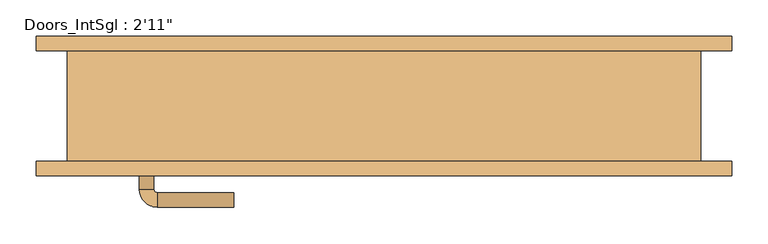
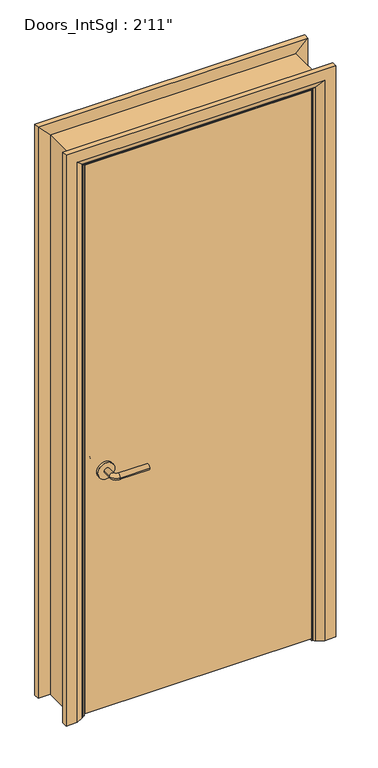
"""IFC4 building model written with IfcOpenShell, lengths in millimetres: door geometry."""

from ifc_helpers import new_model, si_unit, point, frame, frame_2d, origin, place, context, project, spatial, polyline, circle_curve, ellipse_curve, trimmed, segment, composite_curve, outline, extrude, faceted_brep, source, transform, mapped, element, save
from ifc_brep_helpers import plane_surface, cylinder_surface, revolved_surface, advanced_brep


def door_526ed47c(model_context):
    return source(origin(), model_context, "Body", "SolidModel", [
        advanced_brep(
        [(-337.5, -30.2, 900.0), (-317.5, -30.2, 900.0), (-337.5, -0.2, 900.0), (-317.5, -0.2, 900.0), (-312.5, 4.8, 900.0), (-312.5, 24.8, 900.0), (-207.5, 24.8, 900.0), (-207.5, 4.8, 900.0)],
        [
            (0, 1, circle_curve(frame((-327.5, -30.2, 900.0), z_axis=(0.0, -1.0, 0.0), x_axis=(1.0, 0.0, 0.0)), 10.0)),
            (1, 0, circle_curve(frame((-327.5, -30.2, 900.0), z_axis=(0.0, -1.0, 0.0), x_axis=(1.0, 0.0, 0.0)), 10.0)),
            (0, 2),
            (2, 3, circle_curve(frame((-327.5, -0.2, 900.0), z_axis=(0.0, -1.0, 0.0), x_axis=(1.0, 0.0, 0.0)), 10.0)),
            (3, 1),
            (3, 2, circle_curve(frame((-327.5, -0.2, 900.0), z_axis=(0.0, -1.0, 0.0), x_axis=(1.0, 0.0, 0.0)), 10.0)),
            (4, 3, circle_curve(frame((-312.5, -0.2, 900.0), z_axis=(0.0, 0.0, 1.0), x_axis=(-1.0, 0.0, 0.0)), 5.0)),
            (2, 5, circle_curve(frame((-312.5, -0.2, 900.0), z_axis=(0.0, 0.0, -1.0), x_axis=(-1.0, 0.0, 0.0)), 25.0)),
            (5, 4, circle_curve(frame((-312.5, 14.8, 900.0), z_axis=(-1.0, 0.0, 0.0), x_axis=(0.0, -1.0, 0.0)), 10.0)),
            (4, 5, circle_curve(frame((-312.5, 14.8, 900.0), z_axis=(-1.0, 0.0, 0.0), x_axis=(0.0, -1.0, 0.0)), 10.0)),
            (6, 7, circle_curve(frame((-207.5, 14.8, 900.0), z_axis=(1.0, 0.0, 0.0), x_axis=(0.0, -1.0, 0.0)), 10.0)),
            (7, 6, circle_curve(frame((-207.5, 14.8, 900.0), z_axis=(1.0, 0.0, 0.0), x_axis=(0.0, -1.0, 0.0)), 10.0)),
            (5, 6),
            (7, 4),
        ],
        [
            plane_surface(frame((-327.5, -30.2, 900.0), z_axis=(0.0, -1.0, 0.0), x_axis=(0.0, 0.0, 1.0))),
            cylinder_surface(frame((-327.5, -30.2, 900.0), z_axis=(0.0, -1.0, 0.0), x_axis=(1.0, 0.0, 0.0)), 10.0),
            revolved_surface(trimmed(ellipse_curve(frame((-327.5, -0.2, 900.0), z_axis=(0.0, -1.0, 0.0), x_axis=(1.0, 0.0, 0.0)), 10.0, 10.0), [point((-337.5, -0.2, 900.0))], [point((-317.5, -0.2, 900.0))], True, "CARTESIAN"), (-312.5, -0.2, 900.0), (0.0, 0.0, -1.0)),
            revolved_surface(trimmed(ellipse_curve(frame((-327.5, -0.2, 900.0), z_axis=(0.0, -1.0, 0.0), x_axis=(1.0, 0.0, 0.0)), 10.0, 10.0), [point((-317.5, -0.2, 900.0))], [point((-337.5, -0.2, 900.0))], True, "CARTESIAN"), (-312.5, -0.2, 900.0), (0.0, 0.0, -1.0)),
            plane_surface(frame((-207.5, 14.8, 900.0), z_axis=(1.0, 0.0, 0.0), x_axis=(0.0, 0.0, 1.0))),
            cylinder_surface(frame((-312.5, 14.8, 900.0), z_axis=(-1.0, 0.0, 0.0), x_axis=(0.0, -1.0, 0.0)), 10.0),
        ],
        [
            (0, [[1, 2]]),
            (1, [[-1, 3, 4, 5]]),
            (1, [[-2, -5, 6, -3]]),
            (2, [[7, -4, 8, 9]]),
            (3, [[-8, -6, -7, 10]]),
            (4, [[11, 12]]),
            (5, [[-9, 13, -12, 14]]),
            (5, [[-10, -14, -11, -13]]),
        ],
    ),
        extrude(outline(composite_curve([segment(trimmed(circle_curve(frame_2d((900.0, -330.0)), 30.0), [point((900.0, -360.0))], [point((900.0, -300.0))], False, "CARTESIAN"), True, "CONTINUOUS"), segment(trimmed(circle_curve(frame_2d((900.0, -330.0)), 30.0), [point((900.0, -300.0))], [point((900.0, -360.0))], False, "CARTESIAN"), True, "CONTINUOUS")], self_intersect=False)), frame((0.0, -38.2, 0.0), z_axis=(0.0, 1.0, 0.0), x_axis=(0.0, 0.0, 1.0)), (0.0, 0.0, 1.0), 8.0),
        advanced_brep(
        [(-337.5, -84.2, 900.0), (-317.5, -84.2, 900.0), (-317.5, -114.2, 900.0), (-337.5, -114.2, 900.0), (-312.5, -119.2, 900.0), (-312.5, -139.2, 900.0), (-207.5, -139.2, 900.0), (-207.5, -119.2, 900.0)],
        [
            (0, 1, circle_curve(frame((-327.5, -84.2, 900.0), z_axis=(0.0, 1.0, 0.0), x_axis=(1.0, 0.0, 0.0)), 10.0)),
            (1, 0, circle_curve(frame((-327.5, -84.2, 900.0), z_axis=(0.0, 1.0, 0.0), x_axis=(1.0, 0.0, 0.0)), 10.0)),
            (1, 2),
            (2, 3, circle_curve(frame((-327.5, -114.2, 900.0), z_axis=(0.0, 1.0, 0.0), x_axis=(1.0, 0.0, 0.0)), 10.0)),
            (3, 0),
            (3, 2, circle_curve(frame((-327.5, -114.2, 900.0), z_axis=(0.0, 1.0, 0.0), x_axis=(1.0, 0.0, 0.0)), 10.0)),
            (4, 5, circle_curve(frame((-312.5, -129.2, 900.0), z_axis=(-1.0, 0.0, 0.0), x_axis=(0.0, 1.0, 0.0)), 10.0)),
            (5, 3, circle_curve(frame((-312.5, -114.2, 900.0), z_axis=(0.0, 0.0, -1.0), x_axis=(-1.0, 0.0, 0.0)), 25.0)),
            (2, 4, circle_curve(frame((-312.5, -114.2, 900.0), z_axis=(0.0, 0.0, 1.0), x_axis=(-1.0, 0.0, 0.0)), 5.0)),
            (5, 4, circle_curve(frame((-312.5, -129.2, 900.0), z_axis=(-1.0, 0.0, 0.0), x_axis=(0.0, 1.0, 0.0)), 10.0)),
            (6, 7, circle_curve(frame((-207.5, -129.2, 900.0), z_axis=(1.0, 0.0, 0.0), x_axis=(0.0, 1.0, 0.0)), 10.0)),
            (7, 6, circle_curve(frame((-207.5, -129.2, 900.0), z_axis=(1.0, 0.0, 0.0), x_axis=(0.0, 1.0, 0.0)), 10.0)),
            (4, 7),
            (6, 5),
        ],
        [
            plane_surface(frame((-327.5, -84.2, 900.0), z_axis=(0.0, 1.0, 0.0), x_axis=(0.0, 0.0, 1.0))),
            cylinder_surface(frame((-327.5, -84.2, 900.0), z_axis=(0.0, 1.0, 0.0), x_axis=(1.0, 0.0, 0.0)), 10.0),
            revolved_surface(trimmed(ellipse_curve(frame((-327.5, -114.2, 900.0), z_axis=(0.0, -1.0, 0.0), x_axis=(1.0, 0.0, 0.0)), 10.0, 10.0), [point((-337.5, -114.2, 900.0))], [point((-317.5, -114.2, 900.0))], True, "CARTESIAN"), (-312.5, -114.2, 900.0), (0.0, 0.0, -1.0)),
            revolved_surface(trimmed(ellipse_curve(frame((-327.5, -114.2, 900.0), z_axis=(0.0, -1.0, 0.0), x_axis=(1.0, 0.0, 0.0)), 10.0, 10.0), [point((-317.5, -114.2, 900.0))], [point((-337.5, -114.2, 900.0))], True, "CARTESIAN"), (-312.5, -114.2, 900.0), (0.0, 0.0, -1.0)),
            plane_surface(frame((-207.5, -129.2, 900.0), z_axis=(1.0, 0.0, 0.0), x_axis=(0.0, 0.0, 1.0))),
            cylinder_surface(frame((-312.5, -129.2, 900.0), z_axis=(-1.0, 0.0, 0.0), x_axis=(0.0, 1.0, 0.0)), 10.0),
        ],
        [
            (0, [[1, 2]]),
            (1, [[3, 4, 5, -2]]),
            (1, [[-5, 6, -3, -1]]),
            (2, [[7, 8, -4, 9]]),
            (3, [[10, -9, -6, -8]]),
            (4, [[11, 12]]),
            (5, [[13, -11, 14, -7]]),
            (5, [[-14, -12, -13, -10]]),
        ],
    ),
        extrude(outline(composite_curve([segment(trimmed(circle_curve(frame_2d((900.0, -330.0)), 30.0), [point((900.0, -360.0))], [point((900.0, -300.0))], False, "CARTESIAN"), True, "CONTINUOUS"), segment(trimmed(circle_curve(frame_2d((900.0, -330.0)), 30.0), [point((900.0, -300.0))], [point((900.0, -360.0))], False, "CARTESIAN"), True, "CONTINUOUS")], self_intersect=False)), frame((0.0, -84.2, 0.0), z_axis=(0.0, 1.0, 0.0), x_axis=(0.0, 0.0, 1.0)), (0.0, 0.0, 1.0), 8.0),
        extrude(outline(polyline([(402.5, -38.2), (402.5, -76.2), (-402.5, -76.2), (-402.5, -38.2), (402.5, -38.2)])), frame((0.0, 0.0, 8.0), z_axis=(0.0, 0.0, 1.0), x_axis=(1.0, 0.0, 0.0)), (0.0, 0.0, 1.0), 2060.0),
        advanced_brep(
        [(479.5, -96.2, 0.0), (439.5, -96.2, 0.0), (413.5, -82.2, 0.0), (409.5, -76.2, 0.0), (479.5, -76.2, 0.0), (479.5, -76.2, 2145.0), (479.5, -96.2, 2145.0), (409.5, -76.2, 2075.0), (-409.5, -76.2, 2075.0), (-409.5, -76.2, 0.0), (-479.5, -76.2, 0.0), (-479.5, -76.2, 2145.0), (413.5, -82.2, 2079.0), (439.5, -96.2, 2105.0), (-479.5, -96.2, 2145.0), (-479.5, -96.2, 0.0), (-439.5, -96.2, 0.0), (-439.5, -96.2, 2105.0), (-413.5, -82.2, 0.0), (-413.5, -82.2, 2079.0)],
        [
            (0, 1),
            (1, 2),
            (2, 3, circle_curve(frame((417.5, -75.2, 0.0), z_axis=(0.0, 0.0, -1.0), x_axis=(1.0, 0.0, 0.0)), 8.0622577)),
            (3, 4),
            (4, 0),
            (4, 5),
            (5, 6),
            (6, 0),
            (3, 7),
            (7, 8),
            (8, 9),
            (9, 10),
            (10, 11),
            (11, 5),
            (2, 12),
            (12, 7, ellipse_curve(frame((417.5, -75.2, 2083.0), z_axis=(0.7071067811865475, 0.0, -0.7071067811865475), x_axis=(-0.7071067811865474, 0.0, -0.7071067811865476)), 11.4017543, 8.0622577)),
            (1, 13),
            (13, 12),
            (6, 14),
            (14, 15),
            (15, 16),
            (16, 17),
            (17, 13),
            (10, 15),
            (14, 11),
            (9, 18, circle_curve(frame((-417.5, -75.2, 0.0), z_axis=(0.0, 0.0, -1.0), x_axis=(-1.0, 0.0, 0.0)), 8.0622577)),
            (18, 16),
            (19, 18),
            (8, 19, ellipse_curve(frame((-417.5, -75.2, 2083.0), z_axis=(-0.7071067811865475, 0.0, -0.7071067811865475), x_axis=(-0.7071067811865474, 0.0, 0.7071067811865476)), 11.4017543, 8.0622577)),
            (19, 17),
            (12, 19),
        ],
        [
            plane_surface(frame((409.5, -76.2, 0.0), z_axis=(0.0, 0.0, -1.0), x_axis=(0.0, 1.0, 0.0))),
            plane_surface(frame((479.5, -96.2, 0.0), z_axis=(1.0, 0.0, 0.0), x_axis=(0.0, 0.0, 1.0))),
            plane_surface(frame((479.5, -76.2, 0.0), z_axis=(0.0, 1.0, 0.0), x_axis=(0.0, 0.0, 1.0))),
            cylinder_surface(frame((417.5, -75.2, 0.0), z_axis=(0.0, 0.0, -1.0), x_axis=(1.0, 0.0, 0.0)), 8.0622577),
            plane_surface(frame((413.5, -82.2, 0.0), z_axis=(-0.4740998230350126, -0.880471099922178, 0.0), x_axis=(0.0, 0.0, 1.0))),
            plane_surface(frame((439.5, -96.2, 0.0), z_axis=(0.0, -1.0, 0.0), x_axis=(0.0, 0.0, 1.0))),
            plane_surface(frame((-479.5, -96.2, 2145.0), z_axis=(-1.0, 0.0, 0.0), x_axis=(0.0, 0.0, -1.0))),
            plane_surface(frame((-409.5, -76.2, 0.0), z_axis=(0.0, 0.0, -1.0), x_axis=(0.0, 1.0, 0.0))),
            cylinder_surface(frame((-417.5, -75.2, 2075.0), z_axis=(0.0, 0.0, 1.0), x_axis=(-1.0, 0.0, 0.0)), 8.0622577),
            plane_surface(frame((-413.5, -82.2, 2079.0), z_axis=(0.47409982303501824, -0.8804710999221749, 0.0), x_axis=(0.0, 0.0, -1.0))),
            plane_surface(frame((479.5, -96.2, 2145.0), z_axis=(0.0, 0.0, 1.0), x_axis=(-1.0, 0.0, 0.0))),
            cylinder_surface(frame((409.5, -75.2, 2083.0), z_axis=(1.0, 0.0, 0.0), x_axis=(0.0, 0.0, 1.0)), 8.0622577),
            plane_surface(frame((413.5, -82.2, 2079.0), z_axis=(0.0, -0.8804710999221764, -0.4740998230350154), x_axis=(-1.0, 0.0, 0.0))),
        ],
        [
            (0, [[1, 2, 3, 4, 5]]),
            (1, [[6, 7, 8, -5]]),
            (2, [[9, 10, 11, 12, 13, 14, -6, -4]]),
            (3, [[15, 16, -9, -3]]),
            (4, [[17, 18, -15, -2]]),
            (5, [[-8, 19, 20, 21, 22, 23, -17, -1]]),
            (6, [[-13, 24, -20, 25]]),
            (7, [[-24, -12, 26, 27, -21]]),
            (8, [[28, -26, -11, 29]]),
            (9, [[-22, -27, -28, 30]]),
            (10, [[-14, -25, -19, -7]]),
            (11, [[31, -29, -10, -16]]),
            (12, [[-23, -30, -31, -18]]),
        ],
    ),
        extrude(outline(polyline([(0.0, -385.5), (2051.0, -385.5), (2051.0, 385.5), (0.0, 385.5), (0.0, 404.5), (2070.0, 404.5), (2070.0, -404.5), (0.0, -404.5), (0.0, -385.5)])), frame((0.0, -36.2, 0.0), z_axis=(0.0, 1.0, 0.0), x_axis=(0.0, 0.0, 1.0)), (0.0, 0.0, 1.0), 32.0),
        advanced_brep(
        [(-479.5, 96.2, 0.0), (-439.5, 96.2, 0.0), (-413.5, 82.2, 0.0), (-409.5, 76.2, 0.0), (-479.5, 76.2, 0.0), (-479.5, 76.2, 2145.0), (-479.5, 96.2, 2145.0), (-409.5, 76.2, 2075.0), (-413.5, 82.2, 2079.0), (-439.5, 96.2, 2105.0), (479.5, 96.2, 0.0), (479.5, 76.2, 0.0), (409.5, 76.2, 0.0), (413.5, 82.2, 0.0), (439.5, 96.2, 0.0), (479.5, 96.2, 2145.0), (439.5, 96.2, 2105.0), (413.5, 82.2, 2079.0), (409.5, 76.2, 2075.0), (479.5, 76.2, 2145.0)],
        [
            (0, 1),
            (1, 2),
            (2, 3, circle_curve(frame((-417.5, 75.2, 0.0), z_axis=(0.0, 0.0, -1.0), x_axis=(-1.0, 0.0, 0.0)), 8.0622577)),
            (3, 4),
            (4, 0),
            (4, 5),
            (5, 6),
            (6, 0),
            (3, 7),
            (7, 5),
            (2, 8),
            (8, 7, ellipse_curve(frame((-417.5, 75.2, 2083.0), z_axis=(-0.7071067811865475, 0.0, -0.7071067811865475), x_axis=(0.7071067811865474, 0.0, -0.7071067811865476)), 11.4017543, 8.0622577)),
            (1, 9),
            (9, 8),
            (6, 9),
            (10, 11),
            (11, 12),
            (12, 13, circle_curve(frame((417.5, 75.2, 0.0), z_axis=(0.0, 0.0, -1.0), x_axis=(1.0, 0.0, 0.0)), 8.0622577)),
            (13, 14),
            (14, 10),
            (15, 10),
            (14, 16),
            (16, 15),
            (13, 17),
            (17, 16),
            (12, 18),
            (18, 17, ellipse_curve(frame((417.5, 75.2, 2083.0), z_axis=(0.7071067811865475, 0.0, -0.7071067811865475), x_axis=(0.7071067811865474, 0.0, 0.7071067811865476)), 11.4017543, 8.0622577)),
            (11, 19),
            (19, 18),
            (15, 19),
            (5, 19),
            (15, 6),
            (7, 18),
            (8, 17),
            (9, 16),
        ],
        [
            plane_surface(frame((-409.5, 149.0010989, 0.0), z_axis=(0.0, 0.0, -1.0), x_axis=(1.0, 0.0, 0.0))),
            plane_surface(frame((-479.5, 96.2, 0.0), z_axis=(-1.0, 0.0, 0.0), x_axis=(0.0, 0.0, 1.0))),
            plane_surface(frame((-479.5, 76.2, 0.0), z_axis=(0.0, -1.0, 0.0), x_axis=(0.0, 0.0, 1.0))),
            cylinder_surface(frame((-417.5, 75.2, 0.0), z_axis=(0.0, 0.0, -1.0), x_axis=(-1.0, 0.0, 0.0)), 8.0622577),
            plane_surface(frame((-413.5, 82.2, 0.0), z_axis=(0.4740998230350183, 0.8804710999221749, 0.0), x_axis=(0.0, 0.0, 1.0))),
            plane_surface(frame((-439.5, 96.2, 0.0), z_axis=(0.0, 1.0, 0.0), x_axis=(0.0, 0.0, 1.0))),
            plane_surface(frame((409.5, 149.0010989, 0.0), z_axis=(0.0, 0.0, -1.0), x_axis=(-1.0, 0.0, 0.0))),
            plane_surface(frame((439.5, 96.2, 2105.0), z_axis=(0.0, 1.0, 0.0), x_axis=(0.0, 0.0, -1.0))),
            plane_surface(frame((413.5, 82.2, 2079.0), z_axis=(-0.4740998230350183, 0.8804710999221749, 0.0), x_axis=(0.0, 0.0, -1.0))),
            cylinder_surface(frame((417.5, 75.2, 2075.0), z_axis=(0.0, 0.0, 1.0), x_axis=(1.0, 0.0, 0.0)), 8.0622577),
            plane_surface(frame((479.5, 76.2, 2145.0), z_axis=(0.0, -1.0, 0.0), x_axis=(0.0, 0.0, -1.0))),
            plane_surface(frame((479.5, 96.2, 2145.0), z_axis=(1.0, 0.0, 0.0), x_axis=(0.0, 0.0, -1.0))),
            plane_surface(frame((-479.5, 96.2, 2145.0), z_axis=(0.0, 0.0, 1.0), x_axis=(1.0, 0.0, 0.0))),
            plane_surface(frame((-479.5, 76.2, 2145.0), z_axis=(0.0, -1.0, 0.0), x_axis=(1.0, 0.0, 0.0))),
            cylinder_surface(frame((-409.5, 75.2, 2083.0), z_axis=(-1.0, 0.0, 0.0), x_axis=(0.0, 0.0, 1.0)), 8.0622577),
            plane_surface(frame((-413.5, 82.2, 2079.0), z_axis=(0.0, 0.8804710999221749, -0.4740998230350183), x_axis=(1.0, 0.0, 0.0))),
            plane_surface(frame((-439.5, 96.2, 2105.0), z_axis=(0.0, 1.0, 0.0), x_axis=(1.0, 0.0, 0.0))),
        ],
        [
            (0, [[1, 2, 3, 4, 5]]),
            (1, [[6, 7, 8, -5]]),
            (2, [[9, 10, -6, -4]]),
            (3, [[11, 12, -9, -3]]),
            (4, [[13, 14, -11, -2]]),
            (5, [[-8, 15, -13, -1]]),
            (6, [[16, 17, 18, 19, 20]]),
            (7, [[21, -20, 22, 23]]),
            (8, [[-22, -19, 24, 25]]),
            (9, [[-24, -18, 26, 27]]),
            (10, [[-26, -17, 28, 29]]),
            (11, [[-28, -16, -21, 30]]),
            (12, [[31, -30, 32, -7]]),
            (13, [[33, -29, -31, -10]]),
            (14, [[34, -27, -33, -12]]),
            (15, [[35, -25, -34, -14]]),
            (16, [[-32, -23, -35, -15]]),
        ],
    ),
        faceted_brep([(-404.5, -76.2, 0.0), (-436.5, -76.2, 0.0), (-436.5, 76.2, 0.0), (-404.5, 76.2, 0.0), (-404.5, 76.2, 2070.0), (-404.5, -76.2, 2070.0), (-436.5, 76.2, 2102.0), (-436.5, -76.2, 2102.0), (404.5, -76.2, 0.0), (404.5, 76.2, 0.0), (436.5, 76.2, 0.0), (436.5, -76.2, 0.0), (404.5, -76.2, 2070.0), (436.5, -76.2, 2102.0), (436.5, 76.2, 2102.0), (404.5, 76.2, 2070.0)], [[[0, 1, 2, 3]], [[3, 4, 5, 0]], [[2, 6, 4, 3]], [[1, 7, 6, 2]], [[0, 5, 7, 1]], [[8, 9, 10, 11]], [[12, 8, 11, 13]], [[13, 11, 10, 14]], [[14, 10, 9, 15]], [[15, 9, 8, 12]], [[4, 15, 12, 5]], [[6, 14, 15, 4]], [[7, 13, 14, 6]], [[5, 12, 13, 7]]]),
    ])


if __name__ == "__main__":
    model = new_model("IFC4")
    model_context = context("Model", 3, world=origin())
    ifc_project = project(units=[si_unit("LENGTHUNIT", "METRE", prefix="MILLI")], contexts=[model_context])
    site = spatial("IfcSite", under=ifc_project)
    building = spatial("IfcBuilding", under=site)
    placement = place(None, origin())
    door_shape = door_526ed47c(model_context)
    element("IfcDoor", 1, ObjectType="Doors_IntSgl : 2'11\"", at=placement, inside=building, context=model_context, shape_type="MappedRepresentation", body=[
        mapped(door_shape, transform((0.0, 0.0, 0.0), x_axis=(1.0, 0.0, 0.0), y_axis=(0.0, 1.0, 0.0), z_axis=(0.0, 0.0, 1.0))),
    ])
    save(model, "model.ifc")

# Revit data of these elements
# Type "Doors_IntSgl : 2'11\""
#   Type Mark = "48"
#   Type Comments = "Internal Single"
#   Operation = "SingleSwingRight"
#   Manufacturer = "Revit"
#   Keynote = "L20"
#   Description = "Internal Single Door"
#   Analytic Construction = "Metal"
#   UnderCut = 0' - 0.31496"
#   Tolerance = 0' - 0.07874"
#   Thickness = 0' - 1.49606"
#   Thermal Resistance (R) = 0.270117 (m²·K)/W
#   Structural Tolerance = 0' - 0.31496"
#   StopDepth = 0' - 1.25984"
#   Stop Thickness = 0' - 0.74803"
#   Rough Width = 2' - 11"
#   Rough Height = 6' - 11.07087"
#   Height to Top Lock Rail = 3' - 3.37008"
#   Heat Transfer Coefficient (U) = 3.7021 W/(m²·K)
#   Handle Z Distance = 2' - 11.43307"
#   Handle X Distance = 0' - 2.95276"
#   Frame Thickness = 0' - 1.25984"
#   Door Panel Width = 2' - 7.69291"
#   Door Panel Thickness = 0' - 1.49606"
#   Door Panel Offset = 0' - 0"
#   Height = 6' - 11.07087"
#   Width = 2' - 11"
#   Door Panel Height = 6' - 9.10236"
#   Architrave Setback = 0' - 0.19685"
#   Vis - Ironmongery = yes
#   Material Ironmongery = Door - Handle
#   Material Frame = Door - Frame/Mullion (1)
#   Material Door = Door - Panel
#   Material Architrave = Door - Architrave
#   Visual Light Transmittance = 0
#   Solar Heat Gain Coefficient = 0
#   Function = (empty or 0)
#   Wall Closure = (empty or 0)
# Element 1 (IfcDoor, "Doors_IntSgl : 2'11\"")
#   Materials on its faces: "Door - Architrave", "Door - Handle", "Door - Frame/Mullion (1)", "Door - Panel"
# Materials
#   "Door - Handle": colour RGB 0 0 0, transparency 0, Keynote = "P21", Cost = 0
#   "Door - Frame/Mullion (1)": class "Wood", colour RGB 212 179 113, transparency 0, Keynote = "L20", Cost = 0
#   "Door - Panel": class "Wood", colour RGB 210 159 95, transparency 0, Keynote = "L20", Cost = 0
#   "Door - Architrave": class "Wood", colour RGB 154 90 5, transparency 0, Keynote = "P20", Cost = 0
